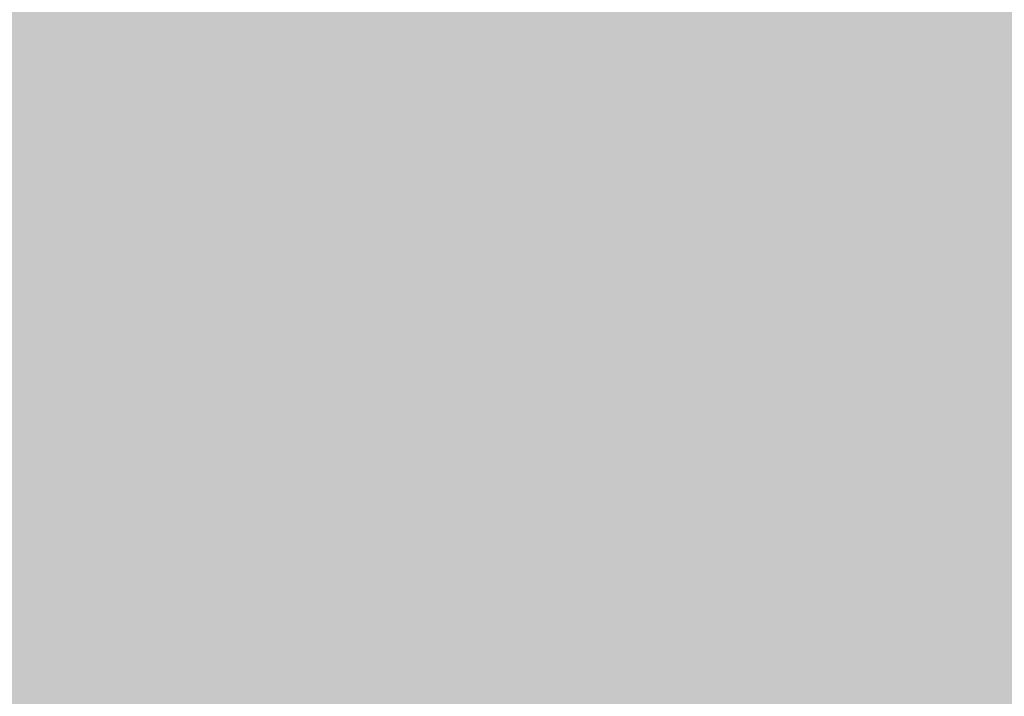
# Model space of a CAD drawing. Units: millimetres. Extents: x 0 to 2267, y 0 to 1823.
# Tile 50 of 256: x 1595.098 to 1596.855, y 1227.321 to 1228.528. Entities that reach past the tile are written whole.
import ezdxf

# ---------------------------------------------------------------- set-up
doc = ezdxf.new("R2010")
doc.units = ezdxf.units.MM
doc.header["$MEASUREMENT"] = 0
doc.layers.add('M-HATC', color=252, linetype='Continuous', lineweight=18)

msp = doc.modelspace()

# ---------------------------------------------------------------- hatches: boundary and pattern name
at = {"layer": 'M-HATC'}
h = msp.add_hatch(color=256, dxfattribs=at)
h.dxf.hatch_style = 1
h.paths.add_polyline_path([(2055.771, 1603.062), (1381.0868, 1603.062), (1381.0868, 1598.062), (2055.771, 1598.062)])
h.paths.add_polyline_path([(2055.771, 1598.062), (1381.0868, 1598.062), (1381.0868, 1593.062), (2055.771, 1593.062)])
h.paths.add_polyline_path([(2051.3074, 1536.7609), (1385.5504, 1536.7609), (1385.5504, 1526.7609), (1387.5504, 1526.7609), (1388.5366, 1525.0528), (1385.3319, 1521.2335), (1385.3319, 1521.2226), (2050.2542, 1522.7491), (2048.3212, 1525.0528), (2049.3074, 1526.7609), (2051.3074, 1526.7609)])
edge = h.paths.add_edge_path()
edge.add_arc((1847.5345, 1379.1492), 135, 222.603061, 222.890851, ccw=False)
edge.add_line((1748.1663, 1287.7656), (1683.0921, 1287.7656))
edge.add_arc((1583.7239, 1379.1492), 135, 317.109149, 317.396939, ccw=False)
edge.add_arc((1678.9686, 1290.6707), 5, 222.8909, 317.1091, ccw=False)
edge.add_arc((1774.2133, 1379.1492), 135, 222.603061, 222.890851, ccw=False)
edge.add_line((1674.8451, 1287.7656), (1609.7709, 1287.7656))
edge.add_arc((1510.4027, 1379.1492), 135, 317.109149, 317.396939, ccw=False)
edge.add_arc((1605.6474, 1290.6707), 5, 222.8909, 317.1091, ccw=False)
edge.add_arc((1700.8921, 1379.1492), 135, 222.603061, 222.890851, ccw=False)
edge.add_line((1601.5239, 1287.7656), (1536.4497, 1287.7656))
edge.add_arc((1437.0815, 1379.1492), 135, 317.109149, 317.396939, ccw=False)
edge.add_arc((1532.3262, 1290.6707), 5, 222.8909, 317.1091, ccw=False)
edge.add_arc((1627.5709, 1379.1492), 135, 222.603061, 222.890851, ccw=False)
edge.add_line((1528.2027, 1287.7656), (1505.9289, 1287.7656))
edge.add_spline(control_points=[(1505.9289, 1287.7656), (1504.2622, 1287.7656), (1504.2622, 1282.7656), (1505.9289, 1282.7656)], knot_values=[0, 0, 0, 0, 5, 5, 5, 5], degree=3, periodic=0)
edge.add_line((1505.9289, 1282.7656), (1930.9289, 1282.7656))
edge.add_spline(control_points=[(1930.9289, 1282.7656), (1932.5956, 1282.7656), (1932.5956, 1287.7656), (1930.9289, 1287.7656)], knot_values=[0, 0, 0, 0, 5, 5, 5, 5], degree=3, periodic=0)
edge.add_line((1930.9289, 1287.7656), (1903.0557, 1287.7656))
edge.add_arc((1803.6875, 1379.1492), 135, 317.109149, 317.396939, ccw=False)
edge.add_arc((1898.9322, 1290.6707), 5, 222.8909, 317.1091, ccw=False)
edge.add_arc((1994.1769, 1379.1492), 135, 222.603061, 222.890851, ccw=False)
edge.add_line((1894.8087, 1287.7656), (1829.7345, 1287.7656))
edge.add_arc((1730.3663, 1379.1492), 135, 317.109149, 317.396939, ccw=False)
edge.add_arc((1825.611, 1290.6707), 5, 222.8909, 317.1091, ccw=False)
edge.add_arc((1920.8557, 1379.1492), 135, 222.603061, 222.890851, ccw=False)
edge.add_line((1821.4875, 1287.7656), (1756.4133, 1287.7656))
edge.add_arc((1657.0451, 1379.1492), 135, 317.109149, 317.396939, ccw=False)
edge.add_arc((1752.2898, 1290.6707), 5, 222.8909, 317.1091, ccw=False)
edge = h.paths.add_edge_path()
edge.add_spline(control_points=[(1843.4289, 1227.2475), (1845.0956, 1227.2475), (1845.0956, 1232.2475), (1843.4289, 1232.2475)], knot_values=[0, 0, 0, 0, 5, 5, 5, 5], degree=3, periodic=0)
edge.add_line((1843.4289, 1232.2475), (1593.4289, 1232.2475))
edge.add_spline(control_points=[(1593.4289, 1232.2475), (1591.7622, 1232.2475), (1591.7622, 1227.2475), (1593.4289, 1227.2475)], knot_values=[0, 0, 0, 0, 5, 5, 5, 5], degree=3, periodic=0)
edge.add_line((1593.4289, 1227.2475), (1843.4289, 1227.2475))
h.paths.add_polyline_path([(1905.9289, 1127.4171), (1530.9289, 1127.4171, 0.414214), (1520.9289, 1117.4171), (1530.9289, 1117.4171), (1915.9289, 1117.4171, 0.414214)])
edge = h.paths.add_edge_path()
edge.add_arc((1397.0858, 1498.4078), 12.7299, 90.78215, 190.87871, ccw=False)
edge.add_line((1396.912, 1511.1365), (1428.0097, 1511.3488))
edge.add_line((1428.0097, 1511.3488), (1433.0097, 1511.3488))
edge.add_line((1433.0097, 1511.3488), (1434.439, 1511.3488))
edge.add_arc((1419.474, 1498.0804), 20, 41.561, 74.08211)
edge.add_line((1424.9592, 1517.3135), (1399.9351, 1517.2561))
edge.add_spline(control_points=[(1399.9307, 1517.2561), (1399.884, 1517.2131), (1399.8328, 1517.1689), (1399.7774, 1517.1236)], knot_values=[11.567499, 11.567499, 11.567499, 11.567499, 11.814249, 11.814249, 11.814249, 11.814249], degree=3, periodic=0)
edge.add_spline(control_points=[(1399.6328, 1517.0099), (1399.5831, 1516.9721), (1399.5307, 1516.9338), (1399.4759, 1516.8947)], knot_values=[11.167718, 11.167718, 11.167718, 11.167718, 11.365188, 11.365188, 11.365188, 11.365188], degree=3, periodic=0)
edge.add_spline(control_points=[(1399.3398, 1516.8001), (1399.1514, 1516.6719), (1398.9384, 1516.5377), (1398.704, 1516.3994)], knot_values=[10.376405, 10.376405, 10.376405, 10.376405, 11.00994, 11.00994, 11.00994, 11.00994], degree=3, periodic=0)
edge.add_spline(control_points=[(1398.6572, 1516.3719), (1398.5789, 1516.326), (1398.4983, 1516.2797), (1398.4155, 1516.2331)], knot_values=[10.125175, 10.125175, 10.125175, 10.125175, 10.334406, 10.334406, 10.334406, 10.334406], degree=3, periodic=0)
edge.add_spline(control_points=[(1398.2642, 1516.1487), (1398.196, 1516.1111), (1398.1263, 1516.0732), (1398.0555, 1516.0351)], knot_values=[9.832246, 9.832246, 9.832246, 9.832246, 9.999658, 9.999658, 9.999658, 9.999658], degree=3, periodic=0)
edge.add_spline(control_points=[(1397.9987, 1516.0048), (1397.7312, 1515.8621), (1397.446, 1515.7171), (1397.1466, 1515.5714)], knot_values=[9.161808, 9.161808, 9.161808, 9.161808, 9.787769, 9.787769, 9.787769, 9.787769], degree=3, periodic=0)
edge.add_spline(control_points=[(1397.1466, 1515.5714), (1396.8418, 1515.423), (1396.5222, 1515.274), (1396.1914, 1515.1262)], knot_values=[8.524455, 8.524455, 8.524455, 8.524455, 9.161808, 9.161808, 9.161808, 9.161808], degree=3, periodic=0)
edge.add_spline(control_points=[(1396.0777, 1515.0756), (1395.9854, 1515.0348), (1395.8922, 1514.994), (1395.7983, 1514.9534)], knot_values=[8.275193, 8.275193, 8.275193, 8.275193, 8.451726, 8.451726, 8.451726, 8.451726], degree=3, periodic=0)
edge.add_spline(control_points=[(1395.6018, 1514.8691), (1395.4997, 1514.8257), (1395.3968, 1514.7824), (1395.2932, 1514.7394)], knot_values=[7.962917, 7.962917, 7.962917, 7.962917, 8.152764, 8.152764, 8.152764, 8.152764], degree=3, periodic=0)
edge.add_spline(control_points=[(1395.2116, 1514.7057), (1394.8278, 1514.5475), (1394.4345, 1514.3929), (1394.0364, 1514.2442)], knot_values=[7.21254, 7.21254, 7.21254, 7.21254, 7.913148, 7.913148, 7.913148, 7.913148], degree=3, periodic=0)
edge.add_spline(control_points=[(1394.0364, 1514.2442), (1393.7076, 1514.1214), (1393.3754, 1514.0027), (1393.0427, 1513.8895)], knot_values=[6.633733, 6.633733, 6.633733, 6.633733, 7.21254, 7.21254, 7.21254, 7.21254], degree=3, periodic=0)
edge.add_spline(control_points=[(1392.8214, 1513.815), (1392.7198, 1513.7812), (1392.6181, 1513.7479), (1392.5166, 1513.7152)], knot_values=[6.328796, 6.328796, 6.328796, 6.328796, 6.505493, 6.505493, 6.505493, 6.505493], degree=3, periodic=0)
edge.add_spline(control_points=[(1392.5166, 1513.7152), (1392.3187, 1513.6515), (1392.1212, 1513.59), (1391.9244, 1513.531)], knot_values=[5.984605, 5.984605, 5.984605, 5.984605, 6.328796, 6.328796, 6.328796, 6.328796], degree=3, periodic=0)
edge.add_spline(control_points=[(1391.7915, 1513.4915), (1391.3122, 1513.3501), (1390.8384, 1513.2239), (1390.3784, 1513.1171)], knot_values=[5.066697, 5.066697, 5.066697, 5.066697, 5.907055, 5.907055, 5.907055, 5.907055], degree=3, periodic=0)
edge.add_spline(control_points=[(1390.3784, 1513.1171), (1390.1797, 1513.071), (1389.9836, 1513.0284), (1389.7907, 1512.9899)], knot_values=[4.70367, 4.70367, 4.70367, 4.70367, 5.066695, 5.066695, 5.066695, 5.066695], degree=3, periodic=0)
edge.add_spline(control_points=[(1389.422, 1512.9204), (1389.2459, 1512.8892), (1389.0729, 1512.8617), (1388.9036, 1512.8381)], knot_values=[4.130571, 4.130571, 4.130571, 4.130571, 4.469816, 4.469816, 4.469816, 4.469816], degree=3, periodic=0)
edge.add_spline(control_points=[(1388.9036, 1512.8381), (1388.591, 1512.7946), (1388.2911, 1512.7644), (1388.0071, 1512.7494)], knot_values=[3.504031, 3.504031, 3.504031, 3.504031, 4.130571, 4.130571, 4.130571, 4.130571], degree=3, periodic=0)
edge.add_spline(control_points=[(1387.9356, 1512.7459), (1387.8538, 1512.7423), (1387.7733, 1512.74), (1387.6944, 1512.739)], knot_values=[3.268866, 3.268866, 3.268866, 3.268866, 3.451164, 3.451164, 3.451164, 3.451164], degree=3, periodic=0)
edge.add_spline(control_points=[(1387.3351, 1512.7443), (1387.2076, 1512.7499), (1387.0847, 1512.7597), (1386.967, 1512.7739)], knot_values=[2.670686, 2.670686, 2.670686, 2.670686, 2.984, 2.984, 2.984, 2.984], degree=3, periodic=0)
edge.add_spline(control_points=[(1386.8327, 1512.7922), (1386.8209, 1512.7941), (1386.8092, 1512.7959), (1386.7975, 1512.7979)], knot_values=[2.516981, 2.516981, 2.516981, 2.516981, 2.549528, 2.549528, 2.549528, 2.549528], degree=3, periodic=0)
edge.add_spline(control_points=[(1386.4526, 1512.8735), (1386.4257, 1512.881), (1386.3993, 1512.889), (1386.3733, 1512.8972)], knot_values=[2.095869, 2.095869, 2.095869, 2.095869, 2.17941, 2.17941, 2.17941, 2.17941], degree=3, periodic=0)
edge.add_spline(control_points=[(1386.0691, 1513.0189), (1386.0634, 1513.0217), (1386.0577, 1513.0246), (1386.052, 1513.0275)], knot_values=[1.72453, 1.72453, 1.72453, 1.72453, 1.745933, 1.745933, 1.745933, 1.745933], degree=3, periodic=0)
edge.add_arc((1399.474, 1498.0804), 20, 131.82432, 180)
edge.add_arc((1630.3336, 1505.5484), 250.9708, 181.705176, 236.427975)
edge.add_arc((1605.3399, 1483.3044), 218.7822, 238.660829, 243.34961)
edge.add_arc((1647.0911, 1510.3592), 262.8986, 183.129836, 237.853442, ccw=False)
h.paths.add_polyline_path([(1406.5369, 1391.9644, 0.149382), (1491.5506, 1296.4418, -0.129517)], flags=17)
edge = h.paths.add_edge_path()
edge.add_arc((2037.3838, 1498.0804), 20, 0, 48.26587)
edge.add_spline(control_points=[(2050.6973, 1513.0052), (2050.6512, 1512.9847), (2050.6034, 1512.9655), (2050.5539, 1512.9477)], knot_values=[1.835652, 1.835652, 1.835652, 1.835652, 2.000781, 2.000781, 2.000781, 2.000781], degree=3, periodic=0)
edge.add_spline(control_points=[(2050.4616, 1512.9166), (2050.479, 1512.9221), (2050.4963, 1512.9277), (2050.5133, 1512.9335)], knot_values=[2.045477, 2.045477, 2.045477, 2.045477, 2.101389, 2.101389, 2.101389, 2.101389], degree=3, periodic=0)
edge.add_spline(control_points=[(2050.129, 1512.8342), (2050.1984, 1512.8473), (2050.2657, 1512.8623), (2050.3308, 1512.8792)], knot_values=[2.237629, 2.237629, 2.237629, 2.237629, 2.435841, 2.435841, 2.435841, 2.435841], degree=3, periodic=0)
edge.add_spline(control_points=[(2050.0946, 1512.8278), (2050.1061, 1512.8299), (2050.1176, 1512.832), (2050.129, 1512.8342)], knot_values=[2.435841, 2.435841, 2.435841, 2.435841, 2.468321, 2.468321, 2.468321, 2.468321], degree=3, periodic=0)
edge.add_spline(control_points=[(2049.7843, 1512.7851), (2049.8552, 1512.7922), (2049.9243, 1512.8008), (2049.9917, 1512.8109)], knot_values=[2.563852, 2.563852, 2.563852, 2.563852, 2.748541, 2.748541, 2.748541, 2.748541], degree=3, periodic=0)
edge.add_spline(control_points=[(2049.4052, 1512.7617), (2049.5364, 1512.7653), (2049.6629, 1512.773), (2049.7843, 1512.7851)], knot_values=[2.748541, 2.748541, 2.748541, 2.748541, 3.064882, 3.064882, 3.064882, 3.064882], degree=3, periodic=0)
edge.add_spline(control_points=[(2049.1698, 1512.7597), (2049.2336, 1512.7591), (2049.2965, 1512.7594), (2049.3584, 1512.7606)], knot_values=[3.102309, 3.102309, 3.102309, 3.102309, 3.2503, 3.2503, 3.2503, 3.2503], degree=3, periodic=0)
edge.add_spline(control_points=[(2048.8573, 1512.7691), (2048.9638, 1512.7638), (2049.068, 1512.7606), (2049.1698, 1512.7597)], knot_values=[3.2503, 3.2503, 3.2503, 3.2503, 3.486069, 3.486069, 3.486069, 3.486069], degree=3, periodic=0)
edge.add_spline(control_points=[(2048.6924, 1512.7789), (2048.3729, 1512.8009), (2048.0345, 1512.8411), (2047.6817, 1512.897)], knot_values=[3.606429, 3.606429, 3.606429, 3.606429, 4.2989, 4.2989, 4.2989, 4.2989], degree=3, periodic=0)
edge.add_spline(control_points=[(2047.6817, 1512.897), (2047.5458, 1512.9185), (2047.4077, 1512.9424), (2047.2678, 1512.9685)], knot_values=[4.2989, 4.2989, 4.2989, 4.2989, 4.565769, 4.565769, 4.565769, 4.565769], degree=3, periodic=0)
edge.add_spline(control_points=[(2047.2678, 1512.9685), (2047.1449, 1512.9914), (2047.0207, 1513.016), (2046.8951, 1513.0422)], knot_values=[4.565769, 4.565769, 4.565769, 4.565769, 4.799971, 4.799971, 4.799971, 4.799971], degree=3, periodic=0)
edge.add_spline(control_points=[(2046.8951, 1513.0422), (2046.5286, 1513.1188), (2046.1513, 1513.209), (2045.7676, 1513.3107)], knot_values=[4.799971, 4.799971, 4.799971, 4.799971, 5.483718, 5.483718, 5.483718, 5.483718], degree=3, periodic=0)
edge.add_spline(control_points=[(2045.7676, 1513.3107), (2045.3724, 1513.4154), (2044.9704, 1513.5322), (2044.5662, 1513.6588)], knot_values=[5.483718, 5.483718, 5.483718, 5.483718, 6.187866, 6.187866, 6.187866, 6.187866], degree=3, periodic=0)
edge.add_spline(control_points=[(2044.5662, 1513.6588), (2044.4149, 1513.7061), (2044.2633, 1513.7549), (2044.1116, 1513.8048)], knot_values=[6.187866, 6.187866, 6.187866, 6.187866, 6.451551, 6.451551, 6.451551, 6.451551], degree=3, periodic=0)
edge.add_spline(control_points=[(2044.1116, 1513.8048), (2043.9967, 1513.8427), (2043.8817, 1513.8813), (2043.7668, 1513.9205)], knot_values=[6.451551, 6.451551, 6.451551, 6.451551, 6.651434, 6.651434, 6.651434, 6.651434], degree=3, periodic=0)
edge.add_spline(control_points=[(2043.7668, 1513.9205), (2043.3716, 1514.0554), (2042.9774, 1514.1979), (2042.5886, 1514.3458)], knot_values=[6.651434, 6.651434, 6.651434, 6.651434, 7.338879, 7.338879, 7.338879, 7.338879], degree=3, periodic=0)
edge.add_spline(control_points=[(2042.5886, 1514.3458), (2042.1643, 1514.5071), (2041.7465, 1514.6749), (2041.3409, 1514.846)], knot_values=[7.338879, 7.338879, 7.338879, 7.338879, 8.089209, 8.089209, 8.089209, 8.089209], degree=3, periodic=0)
edge.add_spline(control_points=[(2041.3409, 1514.846), (2041.1028, 1514.9465), (2040.869, 1515.0481), (2040.6405, 1515.1502)], knot_values=[8.089209, 8.089209, 8.089209, 8.089209, 8.529587, 8.529587, 8.529587, 8.529587], degree=3, periodic=0)
edge.add_spline(control_points=[(2040.51, 1515.2089), (2040.0824, 1515.4022), (2039.6747, 1515.5971), (2039.295, 1515.7894)], knot_values=[8.613818, 8.613818, 8.613818, 8.613818, 9.44571, 9.44571, 9.44571, 9.44571], degree=3, periodic=0)
edge.add_spline(control_points=[(2039.295, 1515.7894), (2039.0618, 1515.9075), (2038.8391, 1516.0246), (2038.6288, 1516.1398)], knot_values=[9.44571, 9.44571, 9.44571, 9.44571, 9.956404, 9.956404, 9.956404, 9.956404], degree=3, periodic=0)
edge.add_spline(control_points=[(2038.6288, 1516.1398), (2038.5187, 1516.2001), (2038.4121, 1516.2598), (2038.309, 1516.3189)], knot_values=[9.956404, 9.956404, 9.956404, 9.956404, 10.223542, 10.223542, 10.223542, 10.223542], degree=3, periodic=0)
edge.add_spline(control_points=[(2038.309, 1516.3189), (2038.2138, 1516.3735), (2038.1216, 1516.4276), (2038.0328, 1516.481)], knot_values=[10.223542, 10.223542, 10.223542, 10.223542, 10.47051, 10.47051, 10.47051, 10.47051], degree=3, periodic=0)
edge.add_spline(control_points=[(2038.0328, 1516.481), (2037.7855, 1516.6296), (2037.5639, 1516.773), (2037.3722, 1516.909)], knot_values=[10.47051, 10.47051, 10.47051, 10.47051, 11.15767, 11.15767, 11.15767, 11.15767], degree=3, periodic=0)
edge.add_spline(control_points=[(2037.3722, 1516.909), (2037.2789, 1516.9752), (2037.1927, 1517.0396), (2037.1142, 1517.102)], knot_values=[11.15767, 11.15767, 11.15767, 11.15767, 11.49227, 11.49227, 11.49227, 11.49227], degree=3, periodic=0)
edge.add_spline(control_points=[(2036.8564, 1517.3259), (2036.9148, 1517.2692), (2036.9814, 1517.2103), (2037.0557, 1517.1492)], knot_values=[11.577341, 11.577341, 11.577341, 11.577341, 11.91035, 11.91035, 11.91035, 11.91035], degree=3, periodic=0)
edge.add_spline(control_points=[(2036.8074, 1517.3748), (2036.823, 1517.3587), (2036.8393, 1517.3424), (2036.8564, 1517.3259)], knot_values=[11.91035, 11.91035, 11.91035, 11.91035, 12.007402, 12.007402, 12.007402, 12.007402], degree=3, periodic=0)
edge.add_spline(control_points=[(2036.7017, 1517.494), (2036.7104, 1517.483), (2036.7196, 1517.4719), (2036.7291, 1517.4606)], knot_values=[12.184155, 12.184155, 12.184155, 12.184155, 12.255409, 12.255409, 12.255409, 12.255409], degree=3, periodic=0)
edge.add_spline(control_points=[(2036.6159, 1517.6205), (2036.62, 1517.613), (2036.6243, 1517.6055), (2036.6289, 1517.5979)], knot_values=[12.487913, 12.487913, 12.487913, 12.487913, 12.541035, 12.541035, 12.541035, 12.541035], degree=3, periodic=0)
edge.add_spline(control_points=[(2036.5635, 1517.786), (2036.5637, 1517.7794), (2036.5642, 1517.7726), (2036.565, 1517.7658)], knot_values=[12.911761, 12.911761, 12.911761, 12.911761, 12.968286, 12.968286, 12.968286, 12.968286], degree=3, periodic=0)
edge.add_spline(control_points=[(2036.6166, 1517.9304), (2036.6125, 1517.9259), (2036.6086, 1517.9212), (2036.6049, 1517.9165)], knot_values=[13.382527, 13.382527, 13.382527, 13.382527, 13.433791, 13.433791, 13.433791, 13.433791], degree=3, periodic=0)
edge.add_spline(control_points=[(2036.749, 1518.017), (2036.7361, 1518.0116), (2036.7239, 1518.006), (2036.7124, 1518.0002)], knot_values=[13.726299, 13.726299, 13.726299, 13.726299, 13.809928, 13.809928, 13.809928, 13.809928], degree=3, periodic=0)
edge.add_spline(control_points=[(2036.8604, 1518.0528), (2036.8386, 1518.0474), (2036.8181, 1518.0416), (2036.7988, 1518.0353)], knot_values=[13.910887, 13.910887, 13.910887, 13.910887, 14.02153, 14.02153, 14.02153, 14.02153], degree=3, periodic=0)
edge.add_line((2036.9639, 1518.0804), (2032.3838, 1518.0804))
edge.add_line((2032.3838, 1518.0804), (2027.3838, 1518.0804))
edge.add_line((2027.3838, 1518.0804), (2022.3838, 1518.0804))
edge.add_line((2022.3838, 1518.0804), (2017.3838, 1518.0804))
edge.add_arc((2017.3838, 1498.0804), 20, 90, 138.439)
edge.add_line((2002.4188, 1511.3488), (2003.8481, 1511.3488))
edge.add_line((2003.8481, 1511.3488), (2008.8481, 1511.3488))
edge.add_line((2008.8481, 1511.3488), (2039.772, 1511.1377))
edge.add_arc((2039.772, 1498.4078), 12.7299, -10.87871, 90, ccw=False)
edge.add_arc((1789.7668, 1510.3592), 262.8986, 302.146558, 356.870164, ccw=False)
edge.add_arc((1831.5179, 1483.3044), 218.7822, 296.65039, 301.339171)
edge.add_arc((1806.5242, 1505.5484), 250.9708, 303.572025, 358.294824)
h.paths.add_polyline_path([(2030.321, 1391.9644, -0.129517), (1945.3072, 1296.4418, 0.149382)], flags=17)
edge = h.paths.add_edge_path()
edge.add_spline(control_points=[(2037.2464, 1518.0821), (2037.2898, 1518.081), (2037.3355, 1518.0804), (2037.3838, 1518.0804)], knot_values=[0.000012, 0.000012, 0.000012, 0.000012, 0.144754, 0.144754, 0.144754, 0.144754], degree=3, periodic=0)
edge.add_line((2037.3357, 1518.0804), (2037.0096, 1518.0804))
edge.add_spline(control_points=[(2037.0096, 1518.0804), (2036.9822, 1518.0768), (2036.956, 1518.0727), (2036.9312, 1518.0681)], knot_values=[14.13465, 14.13465, 14.13465, 14.13465, 14.247197, 14.247197, 14.247197, 14.247197], degree=3, periodic=0)
edge.add_spline(control_points=[(2036.9312, 1518.0681), (2036.9276, 1518.0674), (2036.9241, 1518.0667), (2036.9205, 1518.0661)], knot_values=[14.118315, 14.118315, 14.118315, 14.118315, 14.13465, 14.13465, 14.13465, 14.13465], degree=3, periodic=0)
edge.add_spline(control_points=[(2036.9205, 1518.0661), (2036.9118, 1518.0644), (2036.9032, 1518.0626), (2036.8948, 1518.0608)], knot_values=[14.078086, 14.078086, 14.078086, 14.078086, 14.118315, 14.118315, 14.118315, 14.118315], degree=3, periodic=0)
edge.add_spline(control_points=[(2036.8948, 1518.0608), (2036.883, 1518.0583), (2036.8716, 1518.0556), (2036.8604, 1518.0528)], knot_values=[14.02153, 14.02153, 14.02153, 14.02153, 14.078086, 14.078086, 14.078086, 14.078086], degree=3, periodic=0)
edge.add_spline(control_points=[(2036.8604, 1518.0528), (2036.8386, 1518.0474), (2036.8181, 1518.0416), (2036.7988, 1518.0353)], knot_values=[13.910887, 13.910887, 13.910887, 13.910887, 14.02153, 14.02153, 14.02153, 14.02153], degree=3, periodic=0)
edge.add_spline(control_points=[(2036.7988, 1518.0353), (2036.7981, 1518.035), (2036.7974, 1518.0348), (2036.7967, 1518.0346)], knot_values=[13.906906, 13.906906, 13.906906, 13.906906, 13.910887, 13.910887, 13.910887, 13.910887], degree=3, periodic=0)
edge.add_spline(control_points=[(2036.7967, 1518.0346), (2036.7882, 1518.0318), (2036.7799, 1518.0289), (2036.7719, 1518.0259)], knot_values=[13.857826, 13.857826, 13.857826, 13.857826, 13.906906, 13.906906, 13.906906, 13.906906], degree=3, periodic=0)
edge.add_spline(control_points=[(2036.7719, 1518.0259), (2036.764, 1518.023), (2036.7564, 1518.02), (2036.749, 1518.017)], knot_values=[13.809928, 13.809928, 13.809928, 13.809928, 13.857826, 13.857826, 13.857826, 13.857826], degree=3, periodic=0)
edge.add_spline(control_points=[(2036.749, 1518.017), (2036.7361, 1518.0116), (2036.7239, 1518.006), (2036.7124, 1518.0002)], knot_values=[13.726299, 13.726299, 13.726299, 13.726299, 13.809928, 13.809928, 13.809928, 13.809928], degree=3, periodic=0)
edge.add_spline(control_points=[(2036.7124, 1518.0002), (2036.7121, 1518), (2036.7118, 1517.9999), (2036.7115, 1517.9997)], knot_values=[13.723993, 13.723993, 13.723993, 13.723993, 13.726299, 13.726299, 13.726299, 13.726299], degree=3, periodic=0)
edge.add_spline(control_points=[(2036.7115, 1517.9997), (2036.7063, 1517.9971), (2036.7013, 1517.9944), (2036.6965, 1517.9917)], knot_values=[13.686536, 13.686536, 13.686536, 13.686536, 13.723993, 13.723993, 13.723993, 13.723993], degree=3, periodic=0)
edge.add_spline(control_points=[(2036.6965, 1517.9917), (2036.6919, 1517.9891), (2036.6874, 1517.9865), (2036.6831, 1517.9839)], knot_values=[13.651251, 13.651251, 13.651251, 13.651251, 13.686536, 13.686536, 13.686536, 13.686536], degree=3, periodic=0)
edge.add_spline(control_points=[(2036.6831, 1517.9839), (2036.6764, 1517.9798), (2036.67, 1517.9757), (2036.6639, 1517.9714)], knot_values=[13.596804, 13.596804, 13.596804, 13.596804, 13.651251, 13.651251, 13.651251, 13.651251], degree=3, periodic=0)
edge.add_spline(control_points=[(2036.6639, 1517.9714), (2036.6636, 1517.9712), (2036.6633, 1517.9709), (2036.6629, 1517.9707)], knot_values=[13.593956, 13.593956, 13.593956, 13.593956, 13.596804, 13.596804, 13.596804, 13.596804], degree=3, periodic=0)
edge.add_spline(control_points=[(2036.6629, 1517.9707), (2036.6603, 1517.9689), (2036.6577, 1517.967), (2036.6552, 1517.9651)], knot_values=[13.570322, 13.570322, 13.570322, 13.570322, 13.593956, 13.593956, 13.593956, 13.593956], degree=3, periodic=0)
edge.add_spline(control_points=[(2036.6552, 1517.9651), (2036.6525, 1517.9631), (2036.6499, 1517.9611), (2036.6474, 1517.9591)], knot_values=[13.545477, 13.545477, 13.545477, 13.545477, 13.570322, 13.570322, 13.570322, 13.570322], degree=3, periodic=0)
edge.add_spline(control_points=[(2036.6474, 1517.9591), (2036.6472, 1517.9589), (2036.6471, 1517.9588), (2036.6469, 1517.9587)], knot_values=[13.543931, 13.543931, 13.543931, 13.543931, 13.545477, 13.545477, 13.545477, 13.545477], degree=3, periodic=0)
edge.add_spline(control_points=[(2036.6469, 1517.9587), (2036.6412, 1517.9541), (2036.6358, 1517.9494), (2036.6307, 1517.9447)], knot_values=[13.488237, 13.488237, 13.488237, 13.488237, 13.543931, 13.543931, 13.543931, 13.543931], degree=3, periodic=0)
edge.add_spline(control_points=[(2036.6307, 1517.9447), (2036.6282, 1517.9423), (2036.6257, 1517.9399), (2036.6233, 1517.9374)], knot_values=[13.460307, 13.460307, 13.460307, 13.460307, 13.488237, 13.488237, 13.488237, 13.488237], degree=3, periodic=0)
edge.add_spline(control_points=[(2036.6233, 1517.9374), (2036.6215, 1517.9356), (2036.6198, 1517.9338), (2036.6181, 1517.932)], knot_values=[13.439712, 13.439712, 13.439712, 13.439712, 13.460307, 13.460307, 13.460307, 13.460307], degree=3, periodic=0)
edge.add_spline(control_points=[(2036.6181, 1517.932), (2036.6176, 1517.9315), (2036.6171, 1517.9309), (2036.6166, 1517.9304)], knot_values=[13.433791, 13.433791, 13.433791, 13.433791, 13.439712, 13.439712, 13.439712, 13.439712], degree=3, periodic=0)
edge.add_spline(control_points=[(2036.6166, 1517.9304), (2036.6125, 1517.9259), (2036.6086, 1517.9212), (2036.6049, 1517.9165)], knot_values=[13.382527, 13.382527, 13.382527, 13.382527, 13.433791, 13.433791, 13.433791, 13.433791], degree=3, periodic=0)
edge.add_spline(control_points=[(2036.6049, 1517.9165), (2036.6026, 1517.9135), (2036.6004, 1517.9104), (2036.5982, 1517.9074)], knot_values=[13.350017, 13.350017, 13.350017, 13.350017, 13.382527, 13.382527, 13.382527, 13.382527], degree=3, periodic=0)
edge.add_spline(control_points=[(2036.5982, 1517.9074), (2036.5972, 1517.9059), (2036.5962, 1517.9043), (2036.5952, 1517.9028)], knot_values=[13.333922, 13.333922, 13.333922, 13.333922, 13.350017, 13.350017, 13.350017, 13.350017], degree=3, periodic=0)
edge.add_spline(control_points=[(2036.5952, 1517.9028), (2036.5945, 1517.9018), (2036.5939, 1517.9009), (2036.5933, 1517.8999)], knot_values=[13.323828, 13.323828, 13.323828, 13.323828, 13.333922, 13.333922, 13.333922, 13.333922], degree=3, periodic=0)
edge.add_spline(control_points=[(2036.5933, 1517.8999), (2036.5905, 1517.8955), (2036.5879, 1517.8909), (2036.5855, 1517.8864)], knot_values=[13.277545, 13.277545, 13.277545, 13.277545, 13.323828, 13.323828, 13.323828, 13.323828], degree=3, periodic=0)
edge.add_spline(control_points=[(2036.5855, 1517.8864), (2036.5836, 1517.8827), (2036.5817, 1517.8789), (2036.5801, 1517.8751)], knot_values=[13.240119, 13.240119, 13.240119, 13.240119, 13.277545, 13.277545, 13.277545, 13.277545], degree=3, periodic=0)
edge.add_spline(control_points=[(2036.5801, 1517.8751), (2036.5795, 1517.8739), (2036.579, 1517.8727), (2036.5785, 1517.8715)], knot_values=[13.228211, 13.228211, 13.228211, 13.228211, 13.240119, 13.240119, 13.240119, 13.240119], degree=3, periodic=0)
edge.add_spline(control_points=[(2036.5785, 1517.8715), (2036.578, 1517.8702), (2036.5774, 1517.869), (2036.5769, 1517.8677)], knot_values=[13.215717, 13.215717, 13.215717, 13.215717, 13.228211, 13.228211, 13.228211, 13.228211], degree=3, periodic=0)
edge.add_spline(control_points=[(2036.5769, 1517.8677), (2036.5755, 1517.864), (2036.5741, 1517.8603), (2036.5729, 1517.8565)], knot_values=[13.179847, 13.179847, 13.179847, 13.179847, 13.215717, 13.215717, 13.215717, 13.215717], degree=3, periodic=0)
edge.add_spline(control_points=[(2036.5729, 1517.8565), (2036.5713, 1517.8515), (2036.5699, 1517.8464), (2036.5687, 1517.8413)], knot_values=[13.132017, 13.132017, 13.132017, 13.132017, 13.179847, 13.179847, 13.179847, 13.179847], degree=3, periodic=0)
edge.add_spline(control_points=[(2036.5687, 1517.8413), (2036.5684, 1517.8402), (2036.5682, 1517.8392), (2036.568, 1517.8382)], knot_values=[13.122482, 13.122482, 13.122482, 13.122482, 13.132017, 13.132017, 13.132017, 13.132017], degree=3, periodic=0)
edge.add_spline(control_points=[(2036.568, 1517.8382), (2036.5676, 1517.8363), (2036.5672, 1517.8345), (2036.5669, 1517.8327)], knot_values=[13.105592, 13.105592, 13.105592, 13.105592, 13.122482, 13.122482, 13.122482, 13.122482], degree=3, periodic=0)
edge.add_spline(control_points=[(2036.5669, 1517.8327), (2036.5662, 1517.8292), (2036.5657, 1517.8257), (2036.5652, 1517.8222)], knot_values=[13.074063, 13.074063, 13.074063, 13.074063, 13.105592, 13.105592, 13.105592, 13.105592], degree=3, periodic=0)
edge.add_spline(control_points=[(2036.5652, 1517.8222), (2036.5652, 1517.8222), (2036.5652, 1517.8222), (2036.5652, 1517.8222)], knot_values=[13.074043, 13.074043, 13.074043, 13.074043, 13.074063, 13.074063, 13.074063, 13.074063], degree=3, periodic=0)
edge.add_spline(control_points=[(2036.5652, 1517.8222), (2036.5644, 1517.8164), (2036.5639, 1517.8106), (2036.5636, 1517.8046)], knot_values=[13.021884, 13.021884, 13.021884, 13.021884, 13.074043, 13.074043, 13.074043, 13.074043], degree=3, periodic=0)
edge.add_spline(control_points=[(2036.5636, 1517.8046), (2036.5636, 1517.804), (2036.5636, 1517.8034), (2036.5635, 1517.8028)], knot_values=[13.01674, 13.01674, 13.01674, 13.01674, 13.021884, 13.021884, 13.021884, 13.021884], degree=3, periodic=0)
edge.add_spline(control_points=[(2036.5635, 1517.8028), (2036.5634, 1517.8005), (2036.5634, 1517.7982), (2036.5634, 1517.7958)], knot_values=[12.996438, 12.996438, 12.996438, 12.996438, 13.01674, 13.01674, 13.01674, 13.01674], degree=3, periodic=0)
edge.add_spline(control_points=[(2036.5634, 1517.7958), (2036.5633, 1517.7926), (2036.5634, 1517.7893), (2036.5635, 1517.786)], knot_values=[12.968286, 12.968286, 12.968286, 12.968286, 12.996438, 12.996438, 12.996438, 12.996438], degree=3, periodic=0)
edge.add_spline(control_points=[(2036.5635, 1517.786), (2036.5637, 1517.7794), (2036.5642, 1517.7726), (2036.565, 1517.7658)], knot_values=[12.911761, 12.911761, 12.911761, 12.911761, 12.968286, 12.968286, 12.968286, 12.968286], degree=3, periodic=0)
edge.add_spline(control_points=[(2036.565, 1517.7658), (2036.565, 1517.7657), (2036.565, 1517.7656), (2036.565, 1517.7656)], knot_values=[12.911017, 12.911017, 12.911017, 12.911017, 12.911761, 12.911761, 12.911761, 12.911761], degree=3, periodic=0)
edge.add_spline(control_points=[(2036.565, 1517.7656), (2036.5654, 1517.7625), (2036.5658, 1517.7593), (2036.5663, 1517.7562)], knot_values=[12.88528, 12.88528, 12.88528, 12.88528, 12.911017, 12.911017, 12.911017, 12.911017], degree=3, periodic=0)
edge.add_spline(control_points=[(2036.5663, 1517.7562), (2036.5667, 1517.7534), (2036.5672, 1517.7506), (2036.5677, 1517.7478)], knot_values=[12.862519, 12.862519, 12.862519, 12.862519, 12.88528, 12.88528, 12.88528, 12.88528], degree=3, periodic=0)
edge.add_spline(control_points=[(2036.5677, 1517.7478), (2036.5678, 1517.7474), (2036.5679, 1517.7469), (2036.568, 1517.7465)], knot_values=[12.858885, 12.858885, 12.858885, 12.858885, 12.862519, 12.862519, 12.862519, 12.862519], degree=3, periodic=0)
edge.add_spline(control_points=[(2036.568, 1517.7465), (2036.5692, 1517.7399), (2036.5707, 1517.7332), (2036.5724, 1517.7264)], knot_values=[12.8053, 12.8053, 12.8053, 12.8053, 12.858885, 12.858885, 12.858885, 12.858885], degree=3, periodic=0)
edge.add_spline(control_points=[(2036.5724, 1517.7264), (2036.5734, 1517.7226), (2036.5745, 1517.7187), (2036.5756, 1517.7149)], knot_values=[12.775176, 12.775176, 12.775176, 12.775176, 12.8053, 12.8053, 12.8053, 12.8053], degree=3, periodic=0)
edge.add_spline(control_points=[(2036.5756, 1517.7149), (2036.5763, 1517.7125), (2036.577, 1517.7102), (2036.5778, 1517.7078)], knot_values=[12.756759, 12.756759, 12.756759, 12.756759, 12.775176, 12.775176, 12.775176, 12.775176], degree=3, periodic=0)
edge.add_spline(control_points=[(2036.5778, 1517.7078), (2036.5781, 1517.7067), (2036.5784, 1517.7057), (2036.5787, 1517.7047)], knot_values=[12.748742, 12.748742, 12.748742, 12.748742, 12.756759, 12.756759, 12.756759, 12.756759], degree=3, periodic=0)
edge.add_spline(control_points=[(2036.5787, 1517.7047), (2036.5808, 1517.6983), (2036.5831, 1517.6919), (2036.5856, 1517.6854)], knot_values=[12.69959, 12.69959, 12.69959, 12.69959, 12.748742, 12.748742, 12.748742, 12.748742], degree=3, periodic=0)
edge.add_spline(control_points=[(2036.5856, 1517.6854), (2036.5876, 1517.68), (2036.5898, 1517.6746), (2036.5921, 1517.6692)], knot_values=[12.659038, 12.659038, 12.659038, 12.659038, 12.69959, 12.69959, 12.69959, 12.69959], degree=3, periodic=0)
edge.add_spline(control_points=[(2036.5921, 1517.6692), (2036.594, 1517.6648), (2036.5959, 1517.6605), (2036.5979, 1517.6561)], knot_values=[12.626806, 12.626806, 12.626806, 12.626806, 12.659038, 12.659038, 12.659038, 12.659038], degree=3, periodic=0)
edge.add_spline(control_points=[(2036.5979, 1517.6561), (2036.5984, 1517.6551), (2036.5989, 1517.6541), (2036.5993, 1517.6531)], knot_values=[12.619394, 12.619394, 12.619394, 12.619394, 12.626806, 12.626806, 12.626806, 12.626806], degree=3, periodic=0)
edge.add_spline(control_points=[(2036.5993, 1517.6531), (2036.6043, 1517.6424), (2036.6099, 1517.6315), (2036.6159, 1517.6205)], knot_values=[12.541039, 12.541039, 12.541039, 12.541039, 12.619394, 12.619394, 12.619394, 12.619394], degree=3, periodic=0)
edge.add_spline(control_points=[(2036.6159, 1517.6205), (2036.6159, 1517.6205), (2036.6159, 1517.6205), (2036.6159, 1517.6205)], knot_values=[12.541035, 12.541035, 12.541035, 12.541035, 12.541039, 12.541039, 12.541039, 12.541039], degree=3, periodic=0)
edge.add_spline(control_points=[(2036.6159, 1517.6205), (2036.62, 1517.613), (2036.6243, 1517.6055), (2036.6289, 1517.5979)], knot_values=[12.487913, 12.487913, 12.487913, 12.487913, 12.541035, 12.541035, 12.541035, 12.541035], degree=3, periodic=0)
edge.add_spline(control_points=[(2036.6289, 1517.5979), (2036.6326, 1517.5916), (2036.6365, 1517.5853), (2036.6406, 1517.5789)], knot_values=[12.443982, 12.443982, 12.443982, 12.443982, 12.487913, 12.487913, 12.487913, 12.487913], degree=3, periodic=0)
edge.add_spline(control_points=[(2036.6406, 1517.5789), (2036.6414, 1517.5776), (2036.6423, 1517.5763), (2036.6431, 1517.5749)], knot_values=[12.434996, 12.434996, 12.434996, 12.434996, 12.443982, 12.443982, 12.443982, 12.443982], degree=3, periodic=0)
edge.add_spline(control_points=[(2036.6431, 1517.5749), (2036.6531, 1517.5596), (2036.6639, 1517.5439), (2036.6756, 1517.528)], knot_values=[12.329647, 12.329647, 12.329647, 12.329647, 12.434996, 12.434996, 12.434996, 12.434996], degree=3, periodic=0)
edge.add_spline(control_points=[(2036.6756, 1517.528), (2036.6839, 1517.5168), (2036.6925, 1517.5055), (2036.7017, 1517.494)], knot_values=[12.255409, 12.255409, 12.255409, 12.255409, 12.329647, 12.329647, 12.329647, 12.329647], degree=3, periodic=0)
edge.add_spline(control_points=[(2036.7017, 1517.494), (2036.7104, 1517.483), (2036.7196, 1517.4719), (2036.7291, 1517.4606)], knot_values=[12.184155, 12.184155, 12.184155, 12.184155, 12.255409, 12.255409, 12.255409, 12.255409], degree=3, periodic=0)
edge.add_spline(control_points=[(2036.7291, 1517.4606), (2036.7436, 1517.4435), (2036.759, 1517.4262), (2036.7753, 1517.4085)], knot_values=[12.075961, 12.075961, 12.075961, 12.075961, 12.184155, 12.184155, 12.184155, 12.184155], degree=3, periodic=0)
edge.add_spline(control_points=[(2036.7753, 1517.4085), (2036.7763, 1517.4075), (2036.7773, 1517.4064), (2036.7783, 1517.4054)], knot_values=[12.069502, 12.069502, 12.069502, 12.069502, 12.075961, 12.075961, 12.075961, 12.075961], degree=3, periodic=0)
edge.add_spline(control_points=[(2036.7783, 1517.4054), (2036.7877, 1517.3953), (2036.7974, 1517.385), (2036.8074, 1517.3748)], knot_values=[12.007402, 12.007402, 12.007402, 12.007402, 12.069502, 12.069502, 12.069502, 12.069502], degree=3, periodic=0)
edge.add_spline(control_points=[(2036.8074, 1517.3748), (2036.823, 1517.3587), (2036.8393, 1517.3424), (2036.8564, 1517.3259)], knot_values=[11.91035, 11.91035, 11.91035, 11.91035, 12.007402, 12.007402, 12.007402, 12.007402], degree=3, periodic=0)
edge.add_spline(control_points=[(2036.8564, 1517.3259), (2036.9148, 1517.2692), (2036.9814, 1517.2103), (2037.0557, 1517.1492)], knot_values=[11.577341, 11.577341, 11.577341, 11.577341, 11.91035, 11.91035, 11.91035, 11.91035], degree=3, periodic=0)
edge.add_spline(control_points=[(2037.0557, 1517.1492), (2037.0747, 1517.1336), (2037.0942, 1517.1179), (2037.1142, 1517.102)], knot_values=[11.49227, 11.49227, 11.49227, 11.49227, 11.577341, 11.577341, 11.577341, 11.577341], degree=3, periodic=0)
edge.add_spline(control_points=[(2037.1142, 1517.102), (2037.1927, 1517.0396), (2037.2789, 1516.9752), (2037.3722, 1516.909)], knot_values=[11.15767, 11.15767, 11.15767, 11.15767, 11.49227, 11.49227, 11.49227, 11.49227], degree=3, periodic=0)
edge.add_spline(control_points=[(2037.3722, 1516.909), (2037.5639, 1516.773), (2037.7855, 1516.6296), (2038.0328, 1516.481)], knot_values=[10.47051, 10.47051, 10.47051, 10.47051, 11.15767, 11.15767, 11.15767, 11.15767], degree=3, periodic=0)
edge.add_spline(control_points=[(2038.0328, 1516.481), (2038.1216, 1516.4276), (2038.2138, 1516.3735), (2038.309, 1516.3189)], knot_values=[10.223542, 10.223542, 10.223542, 10.223542, 10.47051, 10.47051, 10.47051, 10.47051], degree=3, periodic=0)
edge.add_spline(control_points=[(2038.309, 1516.3189), (2038.4121, 1516.2598), (2038.5187, 1516.2001), (2038.6288, 1516.1398)], knot_values=[9.956404, 9.956404, 9.956404, 9.956404, 10.223542, 10.223542, 10.223542, 10.223542], degree=3, periodic=0)
edge.add_spline(control_points=[(2038.6288, 1516.1398), (2038.8391, 1516.0246), (2039.0618, 1515.9075), (2039.295, 1515.7894)], knot_values=[9.44571, 9.44571, 9.44571, 9.44571, 9.956404, 9.956404, 9.956404, 9.956404], degree=3, periodic=0)
edge.add_spline(control_points=[(2039.295, 1515.7894), (2039.6747, 1515.5971), (2040.0824, 1515.4022), (2040.51, 1515.2089)], knot_values=[8.613818, 8.613818, 8.613818, 8.613818, 9.44571, 9.44571, 9.44571, 9.44571], degree=3, periodic=0)
edge.add_spline(control_points=[(2040.51, 1515.2089), (2040.5533, 1515.1893), (2040.5968, 1515.1697), (2040.6405, 1515.1502)], knot_values=[8.529587, 8.529587, 8.529587, 8.529587, 8.613818, 8.613818, 8.613818, 8.613818], degree=3, periodic=0)
edge.add_spline(control_points=[(2040.6405, 1515.1502), (2040.869, 1515.0481), (2041.1028, 1514.9465), (2041.3409, 1514.846)], knot_values=[8.089209, 8.089209, 8.089209, 8.089209, 8.529587, 8.529587, 8.529587, 8.529587], degree=3, periodic=0)
edge.add_spline(control_points=[(2041.3409, 1514.846), (2041.7465, 1514.6749), (2042.1643, 1514.5071), (2042.5886, 1514.3458)], knot_values=[7.338879, 7.338879, 7.338879, 7.338879, 8.089209, 8.089209, 8.089209, 8.089209], degree=3, periodic=0)
edge.add_spline(control_points=[(2042.5886, 1514.3458), (2042.9774, 1514.1979), (2043.3716, 1514.0554), (2043.7668, 1513.9205)], knot_values=[6.651434, 6.651434, 6.651434, 6.651434, 7.338879, 7.338879, 7.338879, 7.338879], degree=3, periodic=0)
edge.add_spline(control_points=[(2043.7668, 1513.9205), (2043.8817, 1513.8813), (2043.9967, 1513.8427), (2044.1116, 1513.8048)], knot_values=[6.451551, 6.451551, 6.451551, 6.451551, 6.651434, 6.651434, 6.651434, 6.651434], degree=3, periodic=0)
edge.add_spline(control_points=[(2044.1116, 1513.8048), (2044.2633, 1513.7549), (2044.4149, 1513.7061), (2044.5662, 1513.6588)], knot_values=[6.187866, 6.187866, 6.187866, 6.187866, 6.451551, 6.451551, 6.451551, 6.451551], degree=3, periodic=0)
edge.add_spline(control_points=[(2044.5662, 1513.6588), (2044.9704, 1513.5322), (2045.3724, 1513.4154), (2045.7676, 1513.3107)], knot_values=[5.483718, 5.483718, 5.483718, 5.483718, 6.187866, 6.187866, 6.187866, 6.187866], degree=3, periodic=0)
edge.add_spline(control_points=[(2045.7676, 1513.3107), (2046.1513, 1513.209), (2046.5286, 1513.1188), (2046.8951, 1513.0422)], knot_values=[4.799971, 4.799971, 4.799971, 4.799971, 5.483718, 5.483718, 5.483718, 5.483718], degree=3, periodic=0)
edge.add_spline(control_points=[(2046.8951, 1513.0422), (2047.0207, 1513.016), (2047.1449, 1512.9914), (2047.2678, 1512.9685)], knot_values=[4.565769, 4.565769, 4.565769, 4.565769, 4.799971, 4.799971, 4.799971, 4.799971], degree=3, periodic=0)
edge.add_spline(control_points=[(2047.2678, 1512.9685), (2047.4077, 1512.9424), (2047.5458, 1512.9185), (2047.6817, 1512.897)], knot_values=[4.2989, 4.2989, 4.2989, 4.2989, 4.565769, 4.565769, 4.565769, 4.565769], degree=3, periodic=0)
edge.add_spline(control_points=[(2047.6817, 1512.897), (2048.0345, 1512.8411), (2048.3729, 1512.8009), (2048.6924, 1512.7789)], knot_values=[3.606429, 3.606429, 3.606429, 3.606429, 4.2989, 4.2989, 4.2989, 4.2989], degree=3, periodic=0)
edge.add_spline(control_points=[(2048.6924, 1512.7789), (2048.7479, 1512.7751), (2048.8029, 1512.7718), (2048.8573, 1512.7691)], knot_values=[3.486069, 3.486069, 3.486069, 3.486069, 3.606429, 3.606429, 3.606429, 3.606429], degree=3, periodic=0)
edge.add_spline(control_points=[(2048.8573, 1512.7691), (2048.9638, 1512.7638), (2049.068, 1512.7606), (2049.1698, 1512.7597)], knot_values=[3.2503, 3.2503, 3.2503, 3.2503, 3.486069, 3.486069, 3.486069, 3.486069], degree=3, periodic=0)
edge.add_spline(control_points=[(2049.1698, 1512.7597), (2049.2336, 1512.7591), (2049.2965, 1512.7594), (2049.3584, 1512.7606)], knot_values=[3.102309, 3.102309, 3.102309, 3.102309, 3.2503, 3.2503, 3.2503, 3.2503], degree=3, periodic=0)
edge.add_spline(control_points=[(2049.3584, 1512.7606), (2049.3741, 1512.7609), (2049.3897, 1512.7613), (2049.4052, 1512.7617)], knot_values=[3.064882, 3.064882, 3.064882, 3.064882, 3.102309, 3.102309, 3.102309, 3.102309], degree=3, periodic=0)
edge.add_spline(control_points=[(2049.4052, 1512.7617), (2049.5364, 1512.7653), (2049.6629, 1512.773), (2049.7843, 1512.7851)], knot_values=[2.748541, 2.748541, 2.748541, 2.748541, 3.064882, 3.064882, 3.064882, 3.064882], degree=3, periodic=0)
edge.add_spline(control_points=[(2049.7843, 1512.7851), (2049.8552, 1512.7922), (2049.9243, 1512.8008), (2049.9917, 1512.8109)], knot_values=[2.563852, 2.563852, 2.563852, 2.563852, 2.748541, 2.748541, 2.748541, 2.748541], degree=3, periodic=0)
edge.add_spline(control_points=[(2049.9917, 1512.8109), (2050.0265, 1512.8161), (2050.0608, 1512.8218), (2050.0946, 1512.8278)], knot_values=[2.468321, 2.468321, 2.468321, 2.468321, 2.563852, 2.563852, 2.563852, 2.563852], degree=3, periodic=0)
edge.add_spline(control_points=[(2050.0946, 1512.8278), (2050.1061, 1512.8299), (2050.1176, 1512.832), (2050.129, 1512.8342)], knot_values=[2.435841, 2.435841, 2.435841, 2.435841, 2.468321, 2.468321, 2.468321, 2.468321], degree=3, periodic=0)
edge.add_spline(control_points=[(2050.129, 1512.8342), (2050.1984, 1512.8473), (2050.2657, 1512.8623), (2050.3308, 1512.8792)], knot_values=[2.237629, 2.237629, 2.237629, 2.237629, 2.435841, 2.435841, 2.435841, 2.435841], degree=3, periodic=0)
edge.add_spline(control_points=[(2050.3308, 1512.8792), (2050.3754, 1512.8908), (2050.4191, 1512.9032), (2050.4616, 1512.9166)], knot_values=[2.101389, 2.101389, 2.101389, 2.101389, 2.237629, 2.237629, 2.237629, 2.237629], degree=3, periodic=0)
edge.add_spline(control_points=[(2050.4616, 1512.9166), (2050.479, 1512.9221), (2050.4963, 1512.9277), (2050.5133, 1512.9335)], knot_values=[2.045477, 2.045477, 2.045477, 2.045477, 2.101389, 2.101389, 2.101389, 2.101389], degree=3, periodic=0)
edge.add_spline(control_points=[(2050.5133, 1512.9335), (2050.527, 1512.9382), (2050.5405, 1512.9429), (2050.5539, 1512.9477)], knot_values=[2.000781, 2.000781, 2.000781, 2.000781, 2.045477, 2.045477, 2.045477, 2.045477], degree=3, periodic=0)
edge.add_spline(control_points=[(2050.5539, 1512.9477), (2050.6034, 1512.9655), (2050.6512, 1512.9847), (2050.6973, 1513.0052)], knot_values=[1.835652, 1.835652, 1.835652, 1.835652, 2.000781, 2.000781, 2.000781, 2.000781], degree=3, periodic=0)
edge.add_arc((2037.3838, 1498.0804), 20, 48.26587, 90.12993)
edge = h.paths.add_edge_path(flags=16)
edge.add_spline(control_points=[(1386.1389, 1512.9859), (1388.92, 1511.7395), (1398.0387, 1515.5187), (1399.9307, 1517.2561)], knot_values=[1.831046, 1.831046, 1.831046, 1.831046, 11.814249, 11.814249, 11.814249, 11.814249], degree=3, periodic=0)
edge.add_line((1399.9307, 1517.2561), (1393.7435, 1517.2419))
edge.add_arc((1399.474, 1498.0804), 20, 106.6501, 131.8173)

doc.saveas('drawing.dxf')
